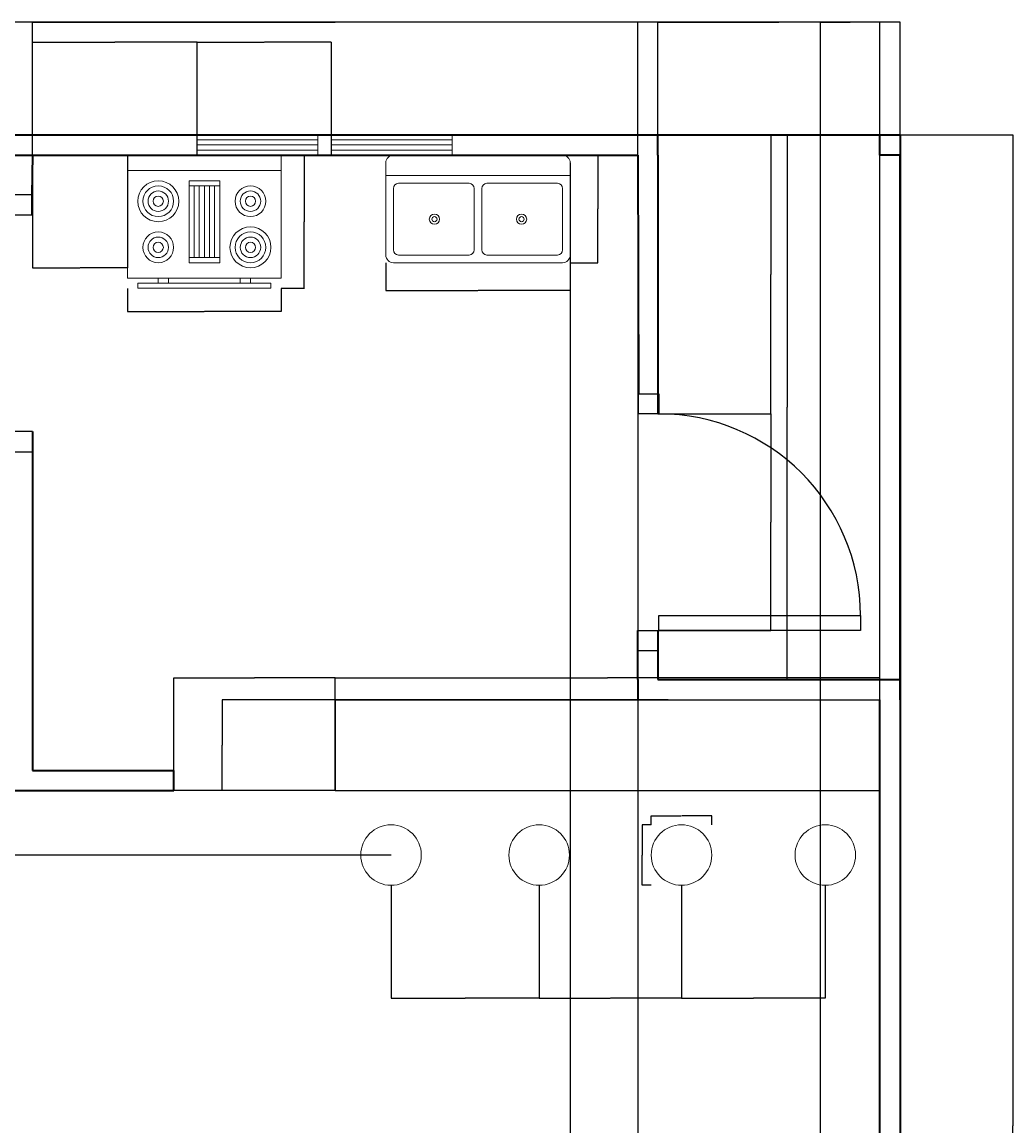
# Model space of a CAD drawing. Units: millimetres. Extents: x 1312 to 12932, y -881 to 10062.
# Tile 4 of 4: x 8020 to 12932, y 4591 to 10062. Entities that reach past the tile are written whole.
import ezdxf

# ---------------------------------------------------------------- set-up
doc = ezdxf.new("R2010")
doc.units = ezdxf.units.MM
for name, color, linetype, lineweight in [('A-ANNO-DIMS', 2, 'Continuous', 18), ('A-DOOR', 3, 'Continuous', 25), ('A-EQPM', 8, 'Continuous', 18), ('A-FLOR-CASE', 32, 'Continuous', 25), ('A-FLOR-FIXT', 9, 'Continuous', 18), ('A-FURN', 8, 'Continuous', 18), ('A-GLAZ', 4, 'Continuous', 18), ('A-WALL', 7, 'Continuous', 35)]:
    doc.layers.add(name, color=color, linetype=linetype, lineweight=lineweight)
doc.styles.get("Standard").update_dxf_attribs({"font": 'arial.ttf'})
doc.dimstyles.get("Standard").update_dxf_attribs({"dimtxt": 0.18, "dimasz": 0.18, "dimexe": 0.18, "dimexo": 0.0625, "dimgap": 0.09, "dimtad": 0, "dimtih": 1, "dimtoh": 1, "dimdec": 4, "dimzin": 0, "dimdsep": 46, "dimtxsty": 'Standard', "dimcen": 0.09, "dimadec": 0, "dimazin": 0, "dimtfac": 1, "dimtdec": 4, "dimtofl": 0, "dimtmove": 0, "dimatfit": 3, "dimfxl": 1, "dimtolj": 1, "dimtzin": 0, "dimarcsym": 0})

# ---------------------------------------------------------------- blocks, each defined once
blk = doc.blocks.new('Range-Oven - 30 in top')
for p, q in [((0, -3), (30, -3)), ((12, -6), (18, -6)), ((13, -20), (13, -6)), ((14, -6), (14, -20)), ((15, -20), (15, -6)), ((16, -6), (16, -20)), ((17, -20), (17, -6)), ((18, -20), (12, -20)), ((6, -24), (6, -25)), ((8, -25), (8, -24)), ((22, -25), (22, -24)), ((24, -24), (24, -25))]:
    blk.add_line(p, q)
for points in [[(0, -24), (0, 0), (30, 0), (30, -24)], [(12, -21), (12, -5), (18, -5), (18, -21)], [(2, -26), (2, -25), (28, -25), (28, -26)]]:
    blk.add_lwpolyline(points, close=True)
for centre, radius in [((6, -9), 4), ((6, -9), 3), ((24, -9), 3), ((6, -9), 2), ((6, -9), 1), ((24, -9), 2), ((24, -9), 1), ((6, -18), 3), ((24, -18), 4), ((24, -18), 3), ((6, -18), 2), ((6, -18), 1), ((24, -18), 2), ((24, -18), 1)]:
    blk.add_circle(centre, radius)
blk = doc.blocks.new('Sink-double - 36 in top')
for p, q in [((-18, -4), (18, -4)), ((-0.75, -18.5), (-0.75, -6.5)), ((0.75, -6.5), (0.75, -18.5))]:
    blk.add_line(p, q)
for points in [[(-16.5, 0), (16.5, 0)], [(-18, -19.5), (-18, -1.5)], [(18, -1.5), (18, -19.5)], [(-15.5, -5.5), (-1.75, -5.5)], [(1.75, -5.5), (15.5, -5.5)], [(-16.5, -18.5), (-16.5, -6.5)], [(16.5, -6.5), (16.5, -18.5)], [(16.5, -21), (-16.5, -21)], [(-1.75, -19.5), (-15.5, -19.5)], [(15.5, -19.5), (1.75, -19.5)]]:
    blk.add_lwpolyline(points)
for centre, radius in [((-8.5, -12.5), 1), ((-8.5, -12.5), 0.5), ((8.5, -12.5), 1), ((8.5, -12.5), 0.5)]:
    blk.add_circle(centre, radius)
for centre, radius, start, end in [((-16.5, -1.5), 1.5, 90, 180), ((16.5, -1.5), 1.5, 0, 90), ((-15.5, -6.5), 1, 90, 180), ((-1.75, -6.5), 1, 0, 90), ((1.75, -6.5), 1, 90, 180), ((15.5, -6.5), 1, 0, 90), ((-15.5, -18.5), 1, 180, 270), ((-1.75, -18.5), 1, 270, 0), ((1.75, -18.5), 1, 180, 270), ((15.5, -18.5), 1, 270, 0), ((-16.5, -19.5), 1.5, 180, 270), ((16.5, -19.5), 1.5, 270, 0)]:
    blk.add_arc(centre, radius, start, end)
blk = doc.blocks.new('Window - Wood Frame 36 in. Wide plan')
for p, q in [((0, 6), (0, 0)), ((0, 4.5), (36, 4.5)), ((36, 6), (36, 0)), ((0, 3), (36, 3)), ((0, 1.5), (36, 1.5))]:
    blk.add_line(p, q)
blk = doc.blocks.new('DOOR-SINGLE-1000')
for p, q in [((0, 1003.8), (0, 1103.8)), ((0, 1103.8), (100, 1103.8)), ((100, 1103.8), (100, 1003.8)), ((1174.2, 1000), (1174.2, 1100)), ((1174.2, 1100), (1274.2, 1100)), ((1274.2, 1100), (1274.2, 1000)), ((100, 1003.8), (0, 1003.8)), ((100, 1000), (174.2, 1000)), ((100, 0), (100, 1000)), ((174.2, 1000), (174.2, 0)), ((1274.2, 1000), (1174.2, 1000)), ((174.2, 0), (100, 0))]:
    blk.add_line(p, q)
blk.add_arc((174.2, 1000), 1000, 270, 0)
blk = doc.blocks.new('STOOL-ROUND-300')
blk.add_circle((150, 150), 150)
blk = doc.blocks.new('*D19')
at = {"layer": 'A-ANNO-DIMS', "color": 0, "lineweight": -2, "transparency": 16777216}
for p, q in [((11138.7, 6083.4), (11138.7, 6128.5)), ((11438.7, 6083.4), (11438.7, 6128.5)), ((11138.9, 6128.3), (11287.7, 6128.3)), ((11438.6, 6128.3), (11289.8, 6128.3))]:
    blk.add_line(p, q, dxfattribs=at)
at = {"layer": 'A-ANNO-DIMS', "color": 0, "transparency": 16777216}
for points in [[(11138.9, 6128.4), (11138.9, 6128.3), (11138.7, 6128.3)], [(11438.6, 6128.4), (11438.6, 6128.3), (11438.7, 6128.3)]]:
    blk.add_solid(points, dxfattribs=at)
at = {"layer": 'Defpoints', "color": 0, "transparency": 16777216}
for p in [(11138.7, 6083.3), (11438.7, 6128.3), (11438.7, 6083.3)]:
    blk.add_point(p, dxfattribs=at)
at = {"layer": 'A-ANNO-DIMS', "color": 0, "transparency": 16777216, "insert": (11288.7, 6128.3), "char_height": 0.18, "attachment_point": 5}
blk.add_mtext('\\A1;STOOL 300 TYP.', dxfattribs=at)
blk = doc.blocks.new('*D20')
at = {"layer": 'A-ANNO-DIMS', "color": 0, "lineweight": -2, "transparency": 16777216}
for p, q in [((11138.7, 6083.3), (11093.6, 6083.3)), ((11093.7, 6083.2), (11093.7, 5933.5)), ((11093.7, 5783.5), (11093.7, 5933.2)), ((11138.7, 5783.3), (11093.6, 5783.3))]:
    blk.add_line(p, q, dxfattribs=at)
at = {"layer": 'A-ANNO-DIMS', "color": 0, "transparency": 16777216}
for points in [[(11093.7, 6083.2), (11093.8, 6083.2), (11093.7, 6083.3)], [(11093.7, 5783.5), (11093.8, 5783.5), (11093.7, 5783.3)]]:
    blk.add_solid(points, dxfattribs=at)
at = {"layer": 'Defpoints', "color": 0, "transparency": 16777216}
for p in [(11093.7, 6083.3), (11138.7, 6083.3), (11138.7, 5783.3)]:
    blk.add_point(p, dxfattribs=at)
at = {"layer": 'A-ANNO-DIMS', "color": 0, "transparency": 16777216, "insert": (11093.7, 5933.3), "char_height": 0.18, "attachment_point": 5}
blk.add_mtext('\\A1;300 TYP.', dxfattribs=at)
blk = doc.blocks.new('*D33')
at = {"layer": 'A-ANNO-DIMS', "color": 0, "lineweight": -2, "transparency": 16777216}
for p, q in [((8542.7, 8742.6), (8542.7, 8628.2)), ((9304.7, 8742.6), (9304.7, 8628.2)), ((8542.9, 8628.4), (8923, 8628.4)), ((9304.5, 8628.4), (8924.5, 8628.4))]:
    blk.add_line(p, q, dxfattribs=at)
at = {"layer": 'A-ANNO-DIMS', "color": 0, "transparency": 16777216}
for points in [[(8542.9, 8628.4), (8542.9, 8628.3), (8542.7, 8628.4)], [(9304.5, 8628.4), (9304.5, 8628.3), (9304.7, 8628.4)]]:
    blk.add_solid(points, dxfattribs=at)
at = {"layer": 'Defpoints', "color": 0, "transparency": 16777216}
for p in [(8542.7, 8742.7), (9304.7, 8742.7), (9304.7, 8628.4)]:
    blk.add_point(p, dxfattribs=at)
at = {"layer": 'A-ANNO-DIMS', "color": 0, "transparency": 16777216, "insert": (8923.7, 8628.4), "char_height": 0.18, "attachment_point": 5}
blk.add_mtext('\\A1;RANGE 762', dxfattribs=at)
blk = doc.blocks.new('*D34')
at = {"layer": 'A-ANNO-DIMS', "color": 0, "lineweight": -2, "transparency": 16777216}
for p, q in [((9304.8, 9403.1), (9419.2, 9403.1)), ((9419, 9402.9), (9419, 9073)), ((9419, 8742.8), (9419, 9072.7)), ((9304.8, 8742.7), (9419.2, 8742.7))]:
    blk.add_line(p, q, dxfattribs=at)
at = {"layer": 'A-ANNO-DIMS', "color": 0, "transparency": 16777216}
for points in [[(9419, 9402.9), (9419, 9402.9), (9419, 9403.1)], [(9419, 8742.8), (9419, 8742.8), (9419, 8742.7)]]:
    blk.add_solid(points, dxfattribs=at)
at = {"layer": 'Defpoints', "color": 0, "transparency": 16777216}
for p in [(9304.7, 9403.1), (9419, 9403.1), (9304.7, 8742.7)]:
    blk.add_point(p, dxfattribs=at)
at = {"layer": 'A-ANNO-DIMS', "color": 0, "transparency": 16777216, "insert": (9419, 9072.9), "char_height": 0.18, "attachment_point": 5}
blk.add_mtext('\\A1;660', dxfattribs=at)
blk = doc.blocks.new('*D35')
at = {"layer": 'A-ANNO-DIMS', "color": 0, "lineweight": -2, "transparency": 16777216}
for p, q in [((9822.8, 8869.6), (9822.8, 8732.3)), ((10737.2, 8869.6), (10737.2, 8732.3)), ((9823, 8732.5), (10278.8, 8732.5)), ((10737, 8732.5), (10281.2, 8732.5))]:
    blk.add_line(p, q, dxfattribs=at)
at = {"layer": 'A-ANNO-DIMS', "color": 0, "transparency": 16777216}
for points in [[(9823, 8732.5), (9823, 8732.5), (9822.8, 8732.5)], [(10737, 8732.5), (10737, 8732.5), (10737.2, 8732.5)]]:
    blk.add_solid(points, dxfattribs=at)
at = {"layer": 'Defpoints', "color": 0, "transparency": 16777216}
for p in [(9822.8, 8869.7), (10737.2, 8869.7), (10737.2, 8732.5)]:
    blk.add_point(p, dxfattribs=at)
at = {"layer": 'A-ANNO-DIMS', "color": 0, "transparency": 16777216, "insert": (10280, 8732.5), "char_height": 0.18, "attachment_point": 5}
blk.add_mtext('\\A1;DOUBLE SINK 914', dxfattribs=at)
blk = doc.blocks.new('*D36')
at = {"layer": 'A-ANNO-DIMS', "color": 0, "lineweight": -2, "transparency": 16777216}
for p, q in [((10737.3, 9403.1), (10874.6, 9403.1)), ((10874.4, 9402.9), (10874.4, 9136.5)), ((10874.4, 8869.8), (10874.4, 9136.2)), ((10737.3, 8869.7), (10874.6, 8869.7))]:
    blk.add_line(p, q, dxfattribs=at)
at = {"layer": 'A-ANNO-DIMS', "color": 0, "transparency": 16777216}
for points in [[(10874.3, 9402.9), (10874.4, 9402.9), (10874.4, 9403.1)], [(10874.3, 8869.8), (10874.4, 8869.8), (10874.4, 8869.7)]]:
    blk.add_solid(points, dxfattribs=at)
at = {"layer": 'Defpoints', "color": 0, "transparency": 16777216}
for p in [(10737.2, 9403.1), (10874.4, 9403.1), (10737.2, 8869.7)]:
    blk.add_point(p, dxfattribs=at)
at = {"layer": 'A-ANNO-DIMS', "color": 0, "transparency": 16777216, "insert": (10874.4, 9136.4), "char_height": 0.18, "attachment_point": 5}
blk.add_mtext('\\A1;533', dxfattribs=at)
blk = doc.blocks.new('*D41')
at = {"layer": 'A-ANNO-DIMS', "color": 0, "lineweight": -2, "transparency": 16777216}
for p, q in [((1872, 9403.1), (1872, 10062.5)), ((1872.2, 10062.3), (7121.6, 10062.3)), ((12371.8, 10062.3), (7122.4, 10062.3)), ((12372, 9503.1), (12372, 10062.5))]:
    blk.add_line(p, q, dxfattribs=at)
at = {"layer": 'A-ANNO-DIMS', "color": 0, "transparency": 16777216}
for points in [[(1872.2, 10062.3), (1872.2, 10062.3), (1872, 10062.3)], [(12371.8, 10062.3), (12371.8, 10062.3), (12372, 10062.3)]]:
    blk.add_solid(points, dxfattribs=at)
at = {"layer": 'Defpoints', "color": 0, "transparency": 16777216}
for p in [(12372, 10062.3), (12372, 9503.1), (1872, 9403.1)]:
    blk.add_point(p, dxfattribs=at)
at = {"layer": 'A-ANNO-DIMS', "color": 0, "transparency": 16777216, "insert": (7122, 10062.3), "char_height": 0.18, "attachment_point": 5}
blk.add_mtext('\\A1;10500', dxfattribs=at)
blk = doc.blocks.new('*D45')
at = {"layer": 'A-ANNO-DIMS', "color": 0, "lineweight": -2, "transparency": 16777216}
for p, q in [((8072, 9403.1), (8072, 10062.5)), ((8072.2, 10062.3), (9571.6, 10062.3)), ((11071.8, 10062.3), (9572.4, 10062.3)), ((11072, 9403.1), (11072, 10062.5))]:
    blk.add_line(p, q, dxfattribs=at)
at = {"layer": 'A-ANNO-DIMS', "color": 0, "transparency": 16777216}
for points in [[(8072.2, 10062.3), (8072.2, 10062.3), (8072, 10062.3)], [(11071.8, 10062.3), (11071.8, 10062.3), (11072, 10062.3)]]:
    blk.add_solid(points, dxfattribs=at)
at = {"layer": 'Defpoints', "color": 0, "transparency": 16777216}
for p in [(11072, 10062.3), (8072, 9403.1), (11072, 9403.1)]:
    blk.add_point(p, dxfattribs=at)
at = {"layer": 'A-ANNO-DIMS', "color": 0, "transparency": 16777216, "insert": (9572, 10062.3), "char_height": 0.18, "attachment_point": 5}
blk.add_mtext('\\A1;3000', dxfattribs=at)
blk = doc.blocks.new('*D46')
at = {"layer": 'A-ANNO-DIMS', "color": 0, "lineweight": -2, "transparency": 16777216}
for p, q in [((11172, 9503.1), (11172, 10062.5)), ((11172.2, 10062.3), (11771.6, 10062.3)), ((12371.8, 10062.3), (11772.3, 10062.3)), ((12372, 9503.1), (12372, 10062.5))]:
    blk.add_line(p, q, dxfattribs=at)
at = {"layer": 'A-ANNO-DIMS', "color": 0, "transparency": 16777216}
for points in [[(11172.2, 10062.3), (11172.2, 10062.3), (11172, 10062.3)], [(12371.8, 10062.3), (12371.8, 10062.3), (12372, 10062.3)]]:
    blk.add_solid(points, dxfattribs=at)
at = {"layer": 'Defpoints', "color": 0, "transparency": 16777216}
for p in [(12372, 10062.3), (11172, 9503.1), (12372, 9503.1)]:
    blk.add_point(p, dxfattribs=at)
at = {"layer": 'A-ANNO-DIMS', "color": 0, "transparency": 16777216, "insert": (11772, 10062.3), "char_height": 0.18, "attachment_point": 5}
blk.add_mtext('\\A1;1200', dxfattribs=at)
blk = doc.blocks.new('*D56')
at = {"layer": 'A-ANNO-DIMS', "color": 0, "lineweight": -2, "transparency": 16777216}
for p, q in [((12371.9, 9503.1), (11812.6, 9503.1)), ((11812.7, 9502.9), (11812.7, 8153.3)), ((11812.7, 6803.3), (11812.7, 8152.9)), ((12371.9, 6803.1), (11812.6, 6803.1))]:
    blk.add_line(p, q, dxfattribs=at)
at = {"layer": 'A-ANNO-DIMS', "color": 0, "transparency": 16777216}
for points in [[(11812.7, 9502.9), (11812.8, 9502.9), (11812.7, 9503.1)], [(11812.7, 6803.3), (11812.8, 6803.3), (11812.7, 6803.1)]]:
    blk.add_solid(points, dxfattribs=at)
at = {"layer": 'Defpoints', "color": 0, "transparency": 16777216}
for p in [(11812.7, 9503.1), (12372, 9503.1), (12372, 6803.1)]:
    blk.add_point(p, dxfattribs=at)
at = {"layer": 'A-ANNO-DIMS', "color": 0, "transparency": 16777216, "insert": (11812.7, 8153.1), "char_height": 0.18, "attachment_point": 5}
blk.add_mtext('\\A1;2700', dxfattribs=at)
blk = doc.blocks.new('*D57')
at = {"layer": 'A-ANNO-DIMS', "color": 0, "lineweight": -2, "transparency": 16777216}
for p, q in [((9571.992231, 6253.123661), (9571.992231, 6812.491161)), ((9572.172231, 6812.311161), (10921.632231, 6812.311161)), ((12271.812231, 6812.311161), (10922.352231, 6812.311161)), ((12271.992231, 6253.123661), (12271.992231, 6812.491161))]:
    blk.add_line(p, q, dxfattribs=at)
at = {"layer": 'A-ANNO-DIMS', "color": 0, "transparency": 16777216}
for points in [[(9572.172231, 6812.341161), (9572.172231, 6812.281161), (9571.992231, 6812.311161)], [(12271.812231, 6812.341161), (12271.812231, 6812.281161), (12271.992231, 6812.311161)]]:
    blk.add_solid(points, dxfattribs=at)
at = {"layer": 'Defpoints', "color": 0, "transparency": 16777216}
for p in [(12271.992231, 6812.311161), (9571.992231, 6253.061161), (12271.992231, 6253.061161)]:
    blk.add_point(p, dxfattribs=at)
at = {"layer": 'A-ANNO-DIMS', "color": 0, "transparency": 16777216, "insert": (10921.992231, 6812.311161), "char_height": 0.18, "attachment_point": 5}
blk.add_mtext('\\A1;2700', dxfattribs=at)
blk = doc.blocks.new('*D58')
at = {"layer": 'A-ANNO-DIMS', "color": 0, "lineweight": -2, "transparency": 16777216}
for p, q in [((9571.9, 6703.1), (9012.6, 6703.1)), ((9012.7, 6702.9), (9012.7, 6478.3)), ((9012.7, 6253.2), (9012.7, 6477.9)), ((9571.9, 6253.1), (9012.6, 6253.1))]:
    blk.add_line(p, q, dxfattribs=at)
at = {"layer": 'A-ANNO-DIMS', "color": 0, "transparency": 16777216}
for points in [[(9012.7, 6702.9), (9012.8, 6702.9), (9012.7, 6703.1)], [(9012.7, 6253.2), (9012.8, 6253.2), (9012.7, 6253.1)]]:
    blk.add_solid(points, dxfattribs=at)
at = {"layer": 'Defpoints', "color": 0, "transparency": 16777216}
for p in [(9012.7, 6703.1), (9572, 6703.1), (9572, 6253.1)]:
    blk.add_point(p, dxfattribs=at)
at = {"layer": 'A-ANNO-DIMS', "color": 0, "transparency": 16777216, "insert": (9012.7, 6478.1), "char_height": 0.18, "attachment_point": 5}
blk.add_mtext('\\A1;450', dxfattribs=at)
blk = doc.blocks.new('*D62')
at = {"layer": 'A-ANNO-DIMS', "color": 0, "lineweight": -2, "transparency": 16777216}
for p, q in [((11172.1, 9503.1), (11731.4, 9503.1)), ((11731.2, 9502.9), (11731.2, 8811.9)), ((11731.2, 8120.5), (11731.2, 8811.5)), ((11172.1, 8120.4), (11731.4, 8120.4))]:
    blk.add_line(p, q, dxfattribs=at)
at = {"layer": 'A-ANNO-DIMS', "color": 0, "transparency": 16777216}
for points in [[(11731.2, 9502.9), (11731.3, 9502.9), (11731.2, 9503.1)], [(11731.2, 8120.5), (11731.3, 8120.5), (11731.2, 8120.4)]]:
    blk.add_solid(points, dxfattribs=at)
at = {"layer": 'Defpoints', "color": 0, "transparency": 16777216}
for p in [(11172, 9503.1), (11172, 8120.4), (11731.2, 8120.4)]:
    blk.add_point(p, dxfattribs=at)
at = {"layer": 'A-ANNO-DIMS', "color": 0, "transparency": 16777216, "insert": (11731.2, 8811.7), "char_height": 0.18, "attachment_point": 5}
blk.add_mtext('\\A1;1382.7', dxfattribs=at)
blk = doc.blocks.new('*D63')
at = {"layer": 'A-ANNO-DIMS', "color": 0, "lineweight": -2, "transparency": 16777216}
for p, q in [((11172.1, 8120.4), (11731.4, 8120.4)), ((11731.2, 8120.2), (11731.2, 7583.4)), ((11731.2, 7046.3), (11731.2, 7583.1)), ((11172.1, 7046.2), (11731.4, 7046.2))]:
    blk.add_line(p, q, dxfattribs=at)
at = {"layer": 'A-ANNO-DIMS', "color": 0, "transparency": 16777216}
for points in [[(11731.2, 8120.2), (11731.3, 8120.2), (11731.2, 8120.4)], [(11731.2, 7046.3), (11731.3, 7046.3), (11731.2, 7046.2)]]:
    blk.add_solid(points, dxfattribs=at)
at = {"layer": 'Defpoints', "color": 0, "transparency": 16777216}
for p in [(11172, 8120.4), (11172, 7046.2), (11731.2, 7046.2)]:
    blk.add_point(p, dxfattribs=at)
at = {"layer": 'A-ANNO-DIMS', "color": 0, "transparency": 16777216, "insert": (11731.2, 7583.3), "char_height": 0.18, "attachment_point": 5}
blk.add_mtext('\\A1;1074.2', dxfattribs=at)
blk = doc.blocks.new('*D67')
at = {"layer": 'A-ANNO-DIMS', "color": 0, "lineweight": -2, "transparency": 16777216}
for p, q in [((8072, 9403.1), (8071.8, 9962.5)), ((8072, 9962.3), (8479.6, 9962.5)), ((8888, 9962.6), (8480.4, 9962.5)), ((8888.4, 9403.4), (8888.2, 9962.8))]:
    blk.add_line(p, q, dxfattribs=at)
at = {"layer": 'A-ANNO-DIMS', "color": 0, "transparency": 16777216}
for points in [[(8072, 9962.3), (8072, 9962.3), (8071.8, 9962.3)], [(8888, 9962.7), (8888, 9962.6), (8888.2, 9962.6)]]:
    blk.add_solid(points, dxfattribs=at)
at = {"layer": 'Defpoints', "color": 0, "transparency": 16777216}
for p in [(8888.2, 9962.6), (8072, 9403.1), (8888.4, 9403.4)]:
    blk.add_point(p, dxfattribs=at)
at = {"layer": 'A-ANNO-DIMS', "color": 0, "transparency": 16777216, "insert": (8480, 9962.5), "char_height": 0.18, "attachment_point": 5}
blk.add_mtext('\\A1;816.4', dxfattribs=at)
blk = doc.blocks.new('*D68')
at = {"layer": 'A-ANNO-DIMS', "color": 0, "lineweight": -2, "transparency": 16777216}
for p, q in [((8888.4, 9403.4), (8888.4, 9962.8)), ((8888.6, 9962.6), (9220.4, 9962.6)), ((9553, 9962.6), (9221.2, 9962.6)), ((9553.2, 9403.4), (9553.2, 9962.8))]:
    blk.add_line(p, q, dxfattribs=at)
at = {"layer": 'A-ANNO-DIMS', "color": 0, "transparency": 16777216}
for points in [[(8888.6, 9962.7), (8888.6, 9962.6), (8888.4, 9962.6)], [(9553, 9962.7), (9553, 9962.6), (9553.2, 9962.6)]]:
    blk.add_solid(points, dxfattribs=at)
at = {"layer": 'Defpoints', "color": 0, "transparency": 16777216}
for p in [(9553.2, 9962.6), (8888.4, 9403.4), (9553.2, 9403.4)]:
    blk.add_point(p, dxfattribs=at)
at = {"layer": 'A-ANNO-DIMS', "color": 0, "transparency": 16777216, "insert": (9220.8, 9962.6), "char_height": 0.18, "attachment_point": 5}
blk.add_mtext('\\A1;664.8', dxfattribs=at)
blk = doc.blocks.new('*D80')
at = {"layer": 'A-ANNO-DIMS', "color": 0, "lineweight": -2, "transparency": 16777216}
for p, q in [((8772, 6253.1), (8772, 6812.5)), ((8772.2, 6812.3), (9171.7, 6812.3)), ((9571.8, 6812.3), (9172.3, 6812.3)), ((9572, 6253.1), (9572, 6812.5))]:
    blk.add_line(p, q, dxfattribs=at)
at = {"layer": 'A-ANNO-DIMS', "color": 0, "transparency": 16777216}
for points in [[(8772.2, 6812.3), (8772.2, 6812.3), (8772, 6812.3)], [(9571.8, 6812.3), (9571.8, 6812.3), (9572, 6812.3)]]:
    blk.add_solid(points, dxfattribs=at)
at = {"layer": 'Defpoints', "color": 0, "transparency": 16777216}
for p in [(9572, 6812.3), (8772, 6253.1), (9572, 6253.1)]:
    blk.add_point(p, dxfattribs=at)
at = {"layer": 'A-ANNO-DIMS', "color": 0, "transparency": 16777216, "insert": (9172, 6812.3), "char_height": 0.18, "attachment_point": 5}
blk.add_mtext('\\A1;800', dxfattribs=at)
blk = doc.blocks.new('*D81')
at = {"layer": 'A-ANNO-DIMS', "color": 0, "lineweight": -2, "transparency": 16777216}
for p, q in [((12372.1, 9503.1), (12931.4, 9503.1)), ((12931.2, 9502.9), (12931.2, 4590.8)), ((12931.2, -321.6), (12931.2, 4590.4)), ((10447.2, -321.8), (12931.4, -321.8))]:
    blk.add_line(p, q, dxfattribs=at)
at = {"layer": 'A-ANNO-DIMS', "color": 0, "transparency": 16777216}
for points in [[(12931.2, 9502.9), (12931.3, 9502.9), (12931.2, 9503.1)], [(12931.2, -321.6), (12931.3, -321.6), (12931.2, -321.8)]]:
    blk.add_solid(points, dxfattribs=at)
at = {"layer": 'Defpoints', "color": 0, "transparency": 16777216}
for p in [(12372, 9503.1), (12931.2, 9503.1), (10447.2, -321.8)]:
    blk.add_point(p, dxfattribs=at)
at = {"layer": 'A-ANNO-DIMS', "color": 0, "transparency": 16777216, "insert": (12931.2, 4590.6), "char_height": 0.18, "attachment_point": 5}
blk.add_mtext('\\A1;9825', dxfattribs=at)
blk = doc.blocks.new('*D89')
at = {"layer": 'A-ANNO-DIMS', "color": 0, "lineweight": -2, "transparency": 16777216}
for p, q in [((8072, 9403), (8072, 8843.6)), ((8542.7, 9403), (8542.7, 8843.6)), ((8072.2, 8843.8), (8307, 8843.8)), ((8542.5, 8843.8), (8307.8, 8843.8))]:
    blk.add_line(p, q, dxfattribs=at)
at = {"layer": 'A-ANNO-DIMS', "color": 0, "transparency": 16777216}
for points in [[(8072.2, 8843.8), (8072.2, 8843.8), (8072, 8843.8)], [(8542.5, 8843.8), (8542.5, 8843.8), (8542.7, 8843.8)]]:
    blk.add_solid(points, dxfattribs=at)
at = {"layer": 'Defpoints', "color": 0, "transparency": 16777216}
for p in [(8072, 9403.1), (8542.7, 9403.1), (8072, 8843.8)]:
    blk.add_point(p, dxfattribs=at)
at = {"layer": 'A-ANNO-DIMS', "color": 0, "transparency": 16777216, "insert": (8307.4, 8843.8), "char_height": 0.18, "attachment_point": 5}
blk.add_mtext('\\A1;470.7', dxfattribs=at)
blk = doc.blocks.new('*D90')
at = {"layer": 'A-ANNO-DIMS', "color": 0, "lineweight": -2, "transparency": 16777216}
for p, q in [((10737.2, 9364.9), (10737.2, -881.3)), ((11072, 9403), (11072, -881.3)), ((10737.4, -881.1), (10904.2, -881.1)), ((11071.8, -881.1), (10905, -881.1))]:
    blk.add_line(p, q, dxfattribs=at)
at = {"layer": 'A-ANNO-DIMS', "color": 0, "transparency": 16777216}
for points in [[(10737.4, -881), (10737.4, -881.1), (10737.2, -881.1)], [(11071.8, -881), (11071.8, -881.1), (11072, -881.1)]]:
    blk.add_solid(points, dxfattribs=at)
at = {"layer": 'Defpoints', "color": 0, "transparency": 16777216}
for p in [(10737.2, 9365), (11072, 9403.1), (11072, -881.1)]:
    blk.add_point(p, dxfattribs=at)
at = {"layer": 'A-ANNO-DIMS', "color": 0, "transparency": 16777216, "insert": (10904.6, -881.1), "char_height": 0.18, "attachment_point": 5}
blk.add_mtext('\\A1;334.8', dxfattribs=at)
blk = doc.blocks.new('*D91')
at = {"layer": 'A-ANNO-DIMS', "color": 0, "lineweight": -2, "transparency": 16777216}
for p, q in [((11288.7, 5783.3), (11288.7, 5223.9)), ((12001.6, 5783.3), (12001.6, 5223.9)), ((11288.9, 5224.1), (11644.8, 5224.1)), ((12001.4, 5224.1), (11645.5, 5224.1))]:
    blk.add_line(p, q, dxfattribs=at)
at = {"layer": 'A-ANNO-DIMS', "color": 0, "transparency": 16777216}
for points in [[(11288.9, 5224.1), (11288.9, 5224.1), (11288.7, 5224.1)], [(12001.4, 5224.1), (12001.4, 5224.1), (12001.6, 5224.1)]]:
    blk.add_solid(points, dxfattribs=at)
at = {"layer": 'Defpoints', "color": 0, "transparency": 16777216}
for p in [(11288.7, 5783.3), (12001.6, 5783.3), (11288.7, 5224.1)]:
    blk.add_point(p, dxfattribs=at)
at = {"layer": 'A-ANNO-DIMS', "color": 0, "transparency": 16777216, "insert": (11645.2, 5224.1), "char_height": 0.18, "attachment_point": 5}
blk.add_mtext('\\A1;712.8', dxfattribs=at)
blk = doc.blocks.new('*D92')
at = {"layer": 'A-ANNO-DIMS', "color": 0, "lineweight": -2, "transparency": 16777216}
for p, q in [((10583, 5783.3), (10583, 5223.9)), ((11288.7, 5783.3), (11288.7, 5223.9)), ((10583.2, 5224.1), (10935.5, 5224.1)), ((11288.6, 5224.1), (10936.3, 5224.1))]:
    blk.add_line(p, q, dxfattribs=at)
at = {"layer": 'A-ANNO-DIMS', "color": 0, "transparency": 16777216}
for points in [[(10583.2, 5224.1), (10583.2, 5224.1), (10583, 5224.1)], [(11288.6, 5224.1), (11288.6, 5224.1), (11288.7, 5224.1)]]:
    blk.add_solid(points, dxfattribs=at)
at = {"layer": 'Defpoints', "color": 0, "transparency": 16777216}
for p in [(10583, 5783.3), (11288.7, 5783.3), (10583, 5224.1)]:
    blk.add_point(p, dxfattribs=at)
at = {"layer": 'A-ANNO-DIMS', "color": 0, "transparency": 16777216, "insert": (10935.9, 5224.1), "char_height": 0.18, "attachment_point": 5}
blk.add_mtext('\\A1;705.8', dxfattribs=at)
blk = doc.blocks.new('*D93')
at = {"layer": 'A-ANNO-DIMS', "color": 0, "lineweight": -2, "transparency": 16777216}
for p, q in [((9849, 5783.3), (9849, 5223.9)), ((10583, 5783.3), (10583, 5223.9)), ((9849.2, 5224.1), (10215.7, 5224.1)), ((10582.8, 5224.1), (10216.3, 5224.1))]:
    blk.add_line(p, q, dxfattribs=at)
at = {"layer": 'A-ANNO-DIMS', "color": 0, "transparency": 16777216}
for points in [[(9849.2, 5224.1), (9849.2, 5224.1), (9849, 5224.1)], [(10582.8, 5224.1), (10582.8, 5224.1), (10583, 5224.1)]]:
    blk.add_solid(points, dxfattribs=at)
at = {"layer": 'Defpoints', "color": 0, "transparency": 16777216}
for p in [(9849, 5783.3), (10583, 5783.3), (9849, 5224.1)]:
    blk.add_point(p, dxfattribs=at)
at = {"layer": 'A-ANNO-DIMS', "color": 0, "transparency": 16777216, "insert": (10216, 5224.1), "char_height": 0.18, "attachment_point": 5}
blk.add_mtext('\\A1;734', dxfattribs=at)
blk = doc.blocks.new('*D94')
at = {"layer": 'A-ANNO-DIMS', "color": 0, "lineweight": -2, "transparency": 16777216}
for p, q in [((9571.9, 6253.1), (1312.6, 6253.1)), ((1312.7, 6252.9), (1312.7, 6093.4)), ((1312.7, 5933.5), (1312.7, 6093)), ((9848.9, 5933.3), (1312.6, 5933.3))]:
    blk.add_line(p, q, dxfattribs=at)
at = {"layer": 'A-ANNO-DIMS', "color": 0, "transparency": 16777216}
for points in [[(1312.7, 6252.9), (1312.8, 6252.9), (1312.7, 6253.1)], [(1312.7, 5933.5), (1312.8, 5933.5), (1312.7, 5933.3)]]:
    blk.add_solid(points, dxfattribs=at)
at = {"layer": 'Defpoints', "color": 0, "transparency": 16777216}
for p in [(1312.7, 6253.1), (9572, 6253.1), (9849, 5933.3)]:
    blk.add_point(p, dxfattribs=at)
at = {"layer": 'A-ANNO-DIMS', "color": 0, "transparency": 16777216, "insert": (1312.7, 6093.2), "char_height": 0.18, "attachment_point": 5}
blk.add_mtext('\\A1;319.7', dxfattribs=at)
blk = doc.blocks.new('*D95')
at = {"layer": 'A-ANNO-DIMS', "color": 0, "lineweight": -2, "transparency": 16777216}
for p, q in [((11977.2, 3005.5), (11977.2, 10062.5)), ((11977.4, 10062.3), (12124.4, 10062.3)), ((12272.1, 10062.3), (12125.1, 10062.3)), ((12272.3, 3024.7), (12272.3, 10062.5))]:
    blk.add_line(p, q, dxfattribs=at)
at = {"layer": 'A-ANNO-DIMS', "color": 0, "transparency": 16777216}
for points in [[(11977.4, 10062.3), (11977.4, 10062.3), (11977.2, 10062.3)], [(12272.1, 10062.3), (12272.1, 10062.3), (12272.3, 10062.3)]]:
    blk.add_solid(points, dxfattribs=at)
at = {"layer": 'Defpoints', "color": 0, "transparency": 16777216}
for p in [(12272.3, 10062.3), (12272.3, 3024.6), (11977.2, 3005.4)]:
    blk.add_point(p, dxfattribs=at)
at = {"layer": 'A-ANNO-DIMS', "color": 0, "transparency": 16777216, "insert": (12124.8, 10062.3), "char_height": 0.18, "attachment_point": 5}
blk.add_mtext('\\A1;295.1', dxfattribs=at)

msp = doc.modelspace()

# ---------------------------------------------------------------- linework, layer by layer
at = {"layer": 'A-FLOR-CASE'}
for p, q in [((9571.992, 6703.088), (11171.992, 6703.088)), ((11221.992, 6703.088), (9571.992, 6703.088)), ((11071.992, 6703.088), (9571.992, 6703.088)), ((9571.992, 6703.088), (9571.992, 6253.061)), ((11171.992, 6703.088), (12271.992, 6703.088)), ((9571.992, 6253.061), (12230.392, 6253.061)), ((12230.392, 6253.061), (12271.992, 6253.061))]:
    msp.add_line(p, q, dxfattribs=at)
at = {"layer": 'A-WALL'}
for p, q in [((1876.635, 9503.061), (12371.992, 9503.061)), ((11171.992, 9403.061), (11171.992, 9503.061)), ((12271.992, 9403.061), (12271.992, 9503.061)), ((12371.992, 9503.061), (12371.992, 9403.061)), ((7968.224, 9403.061), (8071.992, 9403.061)), ((8071.992, 9403.061), (8068.224, 9206.669)), ((8071.992, 9403.061), (11071.992, 9403.061)), ((11071.992, 9403.061), (11075.76, 8220.359)), ((11171.992, 9403.061), (11171.992, 8120.359)), ((11171.992, 9403.061), (11171.992, 8120.359)), ((12371.992, 9403.061), (12271.992, 9403.061)), ((12371.992, 8153.061), (12371.992, 9403.061)), ((12371.992, 9403.061), (12371.992, 1203.088)), ((12371.992, 6703.088), (12371.992, 8153.061)), ((8071.992, 8032.469), (8071.992, 6353.061)), ((8071.992, 8032.469), (8071.992, 6353.061)), ((11071.992, 6803.088), (11071.992, 7046.159)), ((11171.992, 7046.159), (11171.992, 6803.088)), ((11171.992, 7046.159), (11171.992, 6803.088)), ((11071.992, 6803.088), (11071.992, 6703.088)), ((11171.992, 6803.088), (12371.992, 6803.088)), ((11171.992, 6803.088), (11221.992, 6803.088)), ((12271.992, 1303.088), (12271.992, 6703.088)), ((12371.992, 6703.088), (12371.992, 1203.088)), ((8071.992, 6353.061), (8771.992, 6353.061)), ((8771.992, 6253.061), (8771.992, 6353.061)), ((6910.956, 6256.829), (8071.992, 6253.061)), ((8071.992, 6253.061), (8771.992, 6253.061))]:
    msp.add_line(p, q, dxfattribs=at)

# ---------------------------------------------------------------- block references
at = {"layer": 'A-DOOR', "extrusion": (0, 0, -1), "zscale": -1, "rotation": 89.99999999999896}
msp.add_blockref('DOOR-SINGLE-1000', (-6968.224, 7932.468), dxfattribs=at)
at = {"layer": 'A-DOOR', "rotation": 89.99999999999994}
msp.add_blockref('DOOR-SINGLE-1000', (12175.761, 6946.158), dxfattribs=at)
at = {"layer": 'A-EQPM', "xscale": 25.4, "yscale": 25.4, "zscale": 25.4}
msp.add_blockref('Range-Oven - 30 in top', (8542.716, 9403.061), dxfattribs=at)
at = {"layer": 'A-FLOR-FIXT', "xscale": 25.4, "yscale": 25.4, "zscale": 25.4}
msp.add_blockref('Sink-double - 36 in top', (10280.014, 9403.061), dxfattribs=at)
at = {"layer": 'A-FURN'}
for p in [(9698.999, 5783.345), (10432.986, 5783.345), (11138.743, 5783.345), (11851.558, 5783.345)]:
    msp.add_blockref('STOOL-ROUND-300', p, dxfattribs=at)
at = {"layer": 'A-GLAZ', "xscale": 16.61312414671267, "yscale": 16.61312414671267, "zscale": 16.61312414671267}
for p in [(8888.389, 9403.382), (9553.175, 9403.382)]:
    msp.add_blockref('Window - Wood Frame 36 in. Wide plan', p, dxfattribs=at)

# ---------------------------------------------------------------- dimensions: what is measured, and where the dimension line sits
at = {"layer": 'A-ANNO-DIMS'}
for base, p1, p2, override, picture, middle in [((12371.992, 10062.311), (1871.992, 9403.061), (12371.992, 9503.061), {"dimdec": 0, "dimlfac": 1, "dimrnd": 0, "dimzin": 0, "dimdsep": 46, "dimlunit": 2}, '*D41', (7121.992, 10062.311)), ((11071.992, 10062.311), (8071.992, 9403.061), (11071.992, 9403.061), {"dimdec": 0, "dimlfac": 1, "dimrnd": 0, "dimzin": 0, "dimdsep": 46, "dimlunit": 2}, '*D45', (9571.992, 10062.311)), ((12371.992, 10062.311), (11171.992, 9503.061), (12371.992, 9503.061), {"dimdec": 0, "dimlfac": 1, "dimrnd": 0, "dimzin": 0, "dimdsep": 46, "dimlunit": 2}, '*D46', (11771.992, 10062.311)), ((12272.313, 10062.311), (11977.212, 3005.394), (12272.313, 3024.608), {"dimdec": 1, "dimlfac": 1, "dimrnd": 0, "dimzin": 0, "dimdsep": 46, "dimlunit": 2}, '*D95', (12124.763, 10062.311)), ((9553.175, 9962.632), (8888.389, 9403.382), (9553.175, 9403.382), {"dimdec": 1, "dimlfac": 1, "dimrnd": 0, "dimzin": 0, "dimdsep": 46, "dimlunit": 2}, '*D68', (9220.782, 9962.632)), ((11071.992, -881.079), (10737.214, 9364.961), (11071.992, 9403.061), {"dimdec": 1, "dimlfac": 1, "dimrnd": 0, "dimzin": 0, "dimdsep": 46, "dimlunit": 2}, '*D90', (10904.603, -881.079)), ((9571.992, 6812.311), (8771.992, 6253.061), (9571.992, 6253.061), {"dimdec": 0, "dimlfac": 1, "dimrnd": 0, "dimzin": 0, "dimdsep": 46, "dimlunit": 2}, '*D80', (9171.992, 6812.311)), ((12271.992, 6812.311), (9571.992, 6253.061), (12271.992, 6253.061), {"dimdec": 0, "dimlfac": 1, "dimrnd": 0, "dimzin": 0, "dimdsep": 46, "dimlunit": 2}, '*D57', (10921.992, 6812.311))]:
    dim = msp.add_linear_dim(base=base, p1=p1, p2=p2, dimstyle='Standard', override=override, dxfattribs=at)
    dim.commit()
    dim.dimension.update_dxf_attribs({"geometry": picture, "text_midpoint": middle})
for base, p1, p2, angle, override, picture, middle in [((8888.169, 9962.632), (8071.992, 9403.061), (8888.389, 9403.382), 0.022546, {"dimdec": 1, "dimlfac": 1, "dimrnd": 0, "dimzin": 0, "dimdsep": 46, "dimlunit": 2}, '*D67', (8479.97, 9962.472)), ((12931.242, 9503.061), (10447.155, -321.829), (12371.992, 9503.061), 90, {"dimdec": 0, "dimlfac": 1, "dimrnd": 0, "dimzin": 0, "dimdsep": 46, "dimlunit": 2}, '*D81', (12931.242, 4590.616)), ((11731.242, 8120.359), (11171.992, 9503.061), (11171.992, 8120.359), 270, {"dimdec": 1, "dimlfac": 1, "dimrnd": 0, "dimzin": 0, "dimdsep": 46, "dimlunit": 2}, '*D62', (11731.242, 8811.71)), ((11812.742, 9503.061), (12371.992, 6803.088), (12371.992, 9503.061), 90, {"dimdec": 0, "dimlfac": 1, "dimrnd": 0, "dimzin": 0, "dimdsep": 46, "dimlunit": 2}, '*D56', (11812.742, 8153.075)), ((8071.992, 8843.811), (8542.716, 9403.061), (8071.992, 9403.061), 180, {"dimdec": 1, "dimlfac": 1, "dimrnd": 0, "dimzin": 0, "dimdsep": 46, "dimlunit": 2}, '*D89', (8307.354, 8843.811)), ((9419.016, 9403.061), (9304.716, 8742.661), (9304.716, 9403.061), 90, {"dimdec": 0, "dimlfac": 1, "dimrnd": 0, "dimzin": 0, "dimdsep": 46, "dimlunit": 2}, '*D34', (9419.016, 9072.861)), ((10874.374, 9403.061), (10737.214, 8869.661), (10737.214, 9403.061), 90, {"dimdec": 0, "dimlfac": 1, "dimrnd": 0, "dimzin": 0, "dimdsep": 46, "dimlunit": 2}, '*D36', (10874.374, 9136.361)), ((11731.242, 7046.159), (11171.992, 8120.359), (11171.992, 7046.159), 270, {"dimdec": 1, "dimlfac": 1, "dimrnd": 0, "dimzin": 0, "dimdsep": 46, "dimlunit": 2}, '*D63', (11731.242, 7583.259)), ((9012.742, 6703.088), (9571.992, 6253.061), (9571.992, 6703.088), 90, {"dimdec": 0, "dimlfac": 1, "dimrnd": 0, "dimzin": 0, "dimdsep": 46, "dimlunit": 2}, '*D58', (9012.742, 6478.075)), ((1312.742, 6253.061), (9848.999, 5933.345), (9571.992, 6253.061), 90, {"dimdec": 1, "dimlfac": 1, "dimrnd": 0, "dimzin": 0, "dimdsep": 46, "dimlunit": 2}, '*D94', (1312.742, 6093.203)), ((9848.999, 5224.095), (10582.987, 5783.345), (9848.999, 5783.345), 180, {"dimdec": 0, "dimlfac": 1, "dimrnd": 0, "dimzin": 0, "dimdsep": 46, "dimlunit": 2}, '*D93', (10215.993, 5224.095)), ((10582.987, 5224.095), (11288.744, 5783.345), (10582.987, 5783.345), 180, {"dimdec": 1, "dimlfac": 1, "dimrnd": 0, "dimzin": 0, "dimdsep": 46, "dimlunit": 2}, '*D92', (10935.865, 5224.095)), ((11288.744, 5224.095), (12001.559, 5783.345), (11288.744, 5783.345), 180, {"dimdec": 1, "dimlfac": 1, "dimrnd": 0, "dimzin": 0, "dimdsep": 46, "dimlunit": 2}, '*D91', (11645.151, 5224.095))]:
    dim = msp.add_linear_dim(base=base, p1=p1, p2=p2, angle=angle, dimstyle='Standard', override=override, dxfattribs=at)
    dim.commit()
    dim.dimension.update_dxf_attribs({"geometry": picture, "text_midpoint": middle})
for base, p1, p2, text, picture, middle in [((10737.214, 8732.501), (9822.814, 8869.661), (10737.214, 8869.661), 'DOUBLE SINK <>', '*D35', (10280.014, 8732.501)), ((9304.716, 8628.361), (8542.716, 8742.661), (9304.716, 8742.661), 'RANGE <>', '*D33', (8923.716, 8628.361)), ((11438.744, 6128.345), (11138.744, 6083.345), (11438.744, 6083.345), 'STOOL <> TYP.', '*D19', (11288.744, 6128.345))]:
    dim = msp.add_linear_dim(base=base, p1=p1, p2=p2, text=text, dimstyle='Standard', override={"dimdec": 0, "dimlfac": 1, "dimrnd": 0, "dimzin": 0, "dimdsep": 46, "dimlunit": 2}, dxfattribs=at)
    dim.commit()
    dim.dimension.update_dxf_attribs({"geometry": picture, "text_midpoint": middle})
dim = msp.add_linear_dim(base=(11093.744, 6083.345), p1=(11138.744, 5783.345), p2=(11138.744, 6083.345), angle=90, text='<> TYP.', dimstyle='Standard', override={"dimdec": 0, "dimlfac": 1, "dimrnd": 0, "dimzin": 0, "dimdsep": 46, "dimlunit": 2}, dxfattribs=at)
dim.commit()
dim.dimension.update_dxf_attribs({"geometry": '*D20', "text_midpoint": (11093.744, 5933.345)})

doc.saveas('drawing.dxf')
